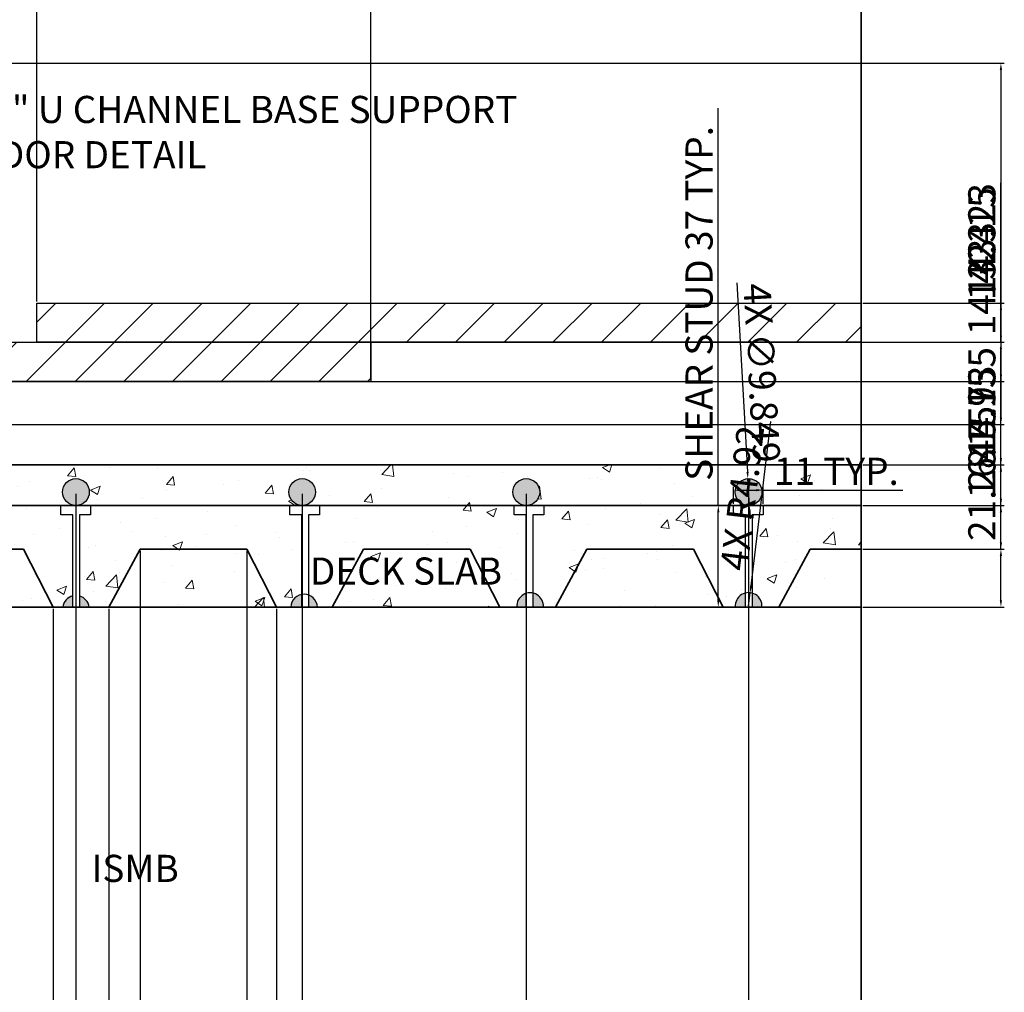
# Model space of a CAD drawing. Units: millimetres. Extents: x 1791 to 2420, y 1225 to 2361.
# Tile 3 of 4: x 2057 to 2420, y 1583 to 1941. Entities that reach past the tile are written whole.
import ezdxf
from ezdxf import colors
from ezdxf.entities.mleader import LeaderData, LeaderLine
from ezdxf.math import Vec2, Vec3

# ---------------------------------------------------------------- set-up
doc = ezdxf.new("R2010")
doc.units = ezdxf.units.MM
for name, color, linetype, lineweight in [('A-ANNO-DIMS', 2, 'Continuous', 18), ('A-ANNO-TEXT', 7, 'Continuous', 18), ('A-ANNO-TTLB', 7, 'Continuous', 35), ('A-DETL-PATT', 8, 'Continuous', 13), ('A-FLOR', 30, 'Continuous', 25), ('S-CONN', 6, 'Continuous', 25), ('S-DECK', 3, 'Continuous', 35)]:
    doc.layers.add(name, color=color, linetype=linetype, lineweight=lineweight)
doc.styles.get("Standard").update_dxf_attribs({"font": 'arial.ttf'})
doc.dimstyles.new('ISO-25', dxfattribs={"dimtxt": 10, "dimasz": 2.5, "dimexe": 1.25, "dimexo": 0.625, "dimtad": 1, "dimdec": 1, "dimtxsty": 'Standard', "dimcen": 2.5, "dimadec": 0, "dimazin": 0, "dimtfac": 1, "dimtdec": 1, "dimtmove": 0, "dimatfit": 3, "dimfxl": 1, "dimarcsym": 0})

# ---------------------------------------------------------------- blocks, each defined once
blk = doc.blocks.new('SHEAR-STUD')
for points in [[(4.38, 33.99), (0, 33.99), (0, 37.44), (10.9, 37.44), (10.9, 33.91), (6.86, 33.91)], [(6.86, 33.91), (6.86, 0), (4.38, 0), (4.38, 33.99)]]:
    blk.add_lwpolyline(points)
blk = doc.blocks.new('*D8')
at = {"layer": 'A-ANNO-DIMS', "color": 0, "lineweight": -2, "transparency": 16777216}
for p, q in [((2314.58, 1762.49), (2314.58, 1908.79)), ((2319.57, 1762.49), (2313.33, 1762.49)), ((2314.58, 1727.56), (2314.58, 1759.99)), ((2319.57, 1725.06), (2313.33, 1725.06))]:
    blk.add_line(p, q, dxfattribs=at)
at = {"layer": 'A-ANNO-DIMS', "color": 0, "transparency": 16777216}
for points in [[(2314.17, 1759.99), (2315, 1759.99), (2314.58, 1762.49)], [(2314.17, 1727.56), (2315, 1727.56), (2314.58, 1725.06)]]:
    blk.add_solid(points, dxfattribs=at)
at = {"layer": 'Defpoints', "color": 0, "transparency": 16777216}
for p in [(2314.58, 1762.49), (2320.2, 1762.49), (2320.2, 1725.06)]:
    blk.add_point(p, dxfattribs=at)
at = {"layer": 'A-ANNO-DIMS', "color": 0, "transparency": 16777216, "insert": (2308.78, 1836.89), "char_height": 10, "attachment_point": 5, "rotation": 90}
blk.add_mtext('SHEAR STUD 37 TYP.', dxfattribs=at)
blk = doc.blocks.new('*D9')
at = {"layer": 'A-ANNO-DIMS', "color": 0, "lineweight": -2, "transparency": 16777216}
for p, q in [((2320.2, 1763.12), (2320.2, 1769.36)), ((2322.7, 1768.11), (2328.6, 1768.11)), ((2331.1, 1763.12), (2331.1, 1769.36)), ((2331.1, 1768.11), (2382.58, 1768.11))]:
    blk.add_line(p, q, dxfattribs=at)
at = {"layer": 'A-ANNO-DIMS', "color": 0, "transparency": 16777216}
for points in [[(2322.7, 1768.52), (2322.7, 1767.69), (2320.2, 1768.11)], [(2328.6, 1768.52), (2328.6, 1767.69), (2331.1, 1768.11)]]:
    blk.add_solid(points, dxfattribs=at)
at = {"layer": 'Defpoints', "color": 0, "transparency": 16777216}
for p in [(2331.1, 1768.11), (2320.2, 1762.49), (2331.1, 1762.49)]:
    blk.add_point(p, dxfattribs=at)
at = {"layer": 'A-ANNO-DIMS', "color": 0, "transparency": 16777216, "insert": (2358.09, 1773.76), "char_height": 10, "attachment_point": 5}
blk.add_mtext('11 TYP.', dxfattribs=at)
blk = doc.blocks.new('*D18')
at = {"layer": 'A-ANNO-DIMS', "color": 0, "lineweight": -2, "transparency": 16777216}
for p, q in [((1926.15, 1925.42), (2419.97, 1925.42)), ((2418.72, 1922.92), (2418.72, 1794.77)), ((1926.15, 1792.27), (2419.97, 1792.27))]:
    blk.add_line(p, q, dxfattribs=at)
at = {"layer": 'A-ANNO-DIMS', "color": 0, "transparency": 16777216}
for points in [[(2418.3, 1922.92), (2419.13, 1922.92), (2418.72, 1925.42)], [(2418.3, 1794.77), (2419.13, 1794.77), (2418.72, 1792.27)]]:
    blk.add_solid(points, dxfattribs=at)
at = {"layer": 'Defpoints', "color": 0, "transparency": 16777216}
for p in [(1925.53, 1925.42), (1925.53, 1792.27), (2418.72, 1792.27)]:
    blk.add_point(p, dxfattribs=at)
at = {"layer": 'A-ANNO-DIMS', "color": 0, "transparency": 16777216, "insert": (2412.98, 1858.85), "char_height": 10, "attachment_point": 5, "rotation": 90}
blk.add_mtext('133.15', dxfattribs=at)
blk = doc.blocks.new('*D19')
at = {"layer": 'A-ANNO-DIMS', "color": 0, "lineweight": -2, "transparency": 16777216}
for p, q in [((2418.72, 1822.58), (2418.72, 1866.9)), ((1941, 1822.58), (2419.97, 1822.58)), ((2418.72, 1810.65), (2418.72, 1820.08)), ((1941, 1808.15), (2419.97, 1808.15))]:
    blk.add_line(p, q, dxfattribs=at)
at = {"layer": 'A-ANNO-DIMS', "color": 0, "transparency": 16777216}
for points in [[(2418.3, 1820.08), (2419.13, 1820.08), (2418.72, 1822.58)], [(2418.3, 1810.65), (2419.13, 1810.65), (2418.72, 1808.15)]]:
    blk.add_solid(points, dxfattribs=at)
at = {"layer": 'Defpoints', "color": 0, "transparency": 16777216}
for p in [(1940.38, 1822.58), (2418.72, 1822.58), (1940.38, 1808.15)]:
    blk.add_point(p, dxfattribs=at)
at = {"layer": 'A-ANNO-DIMS', "color": 0, "transparency": 16777216, "insert": (2412.98, 1845.99), "char_height": 10, "attachment_point": 5, "rotation": 90}
blk.add_mtext('14.423', dxfattribs=at)
blk = doc.blocks.new('*D22')
at = {"layer": 'A-ANNO-DIMS', "color": 0, "lineweight": -2, "transparency": 16777216}
for p, q in [((2418.72, 1746.33), (2418.72, 1784.02)), ((2367.84, 1746.33), (2419.97, 1746.33)), ((2418.72, 1727.56), (2418.72, 1743.83)), ((2367.84, 1725.06), (2419.97, 1725.06))]:
    blk.add_line(p, q, dxfattribs=at)
at = {"layer": 'A-ANNO-DIMS', "color": 0, "transparency": 16777216}
for points in [[(2418.3, 1743.83), (2419.13, 1743.83), (2418.72, 1746.33)], [(2418.3, 1727.56), (2419.13, 1727.56), (2418.72, 1725.06)]]:
    blk.add_solid(points, dxfattribs=at)
at = {"layer": 'Defpoints', "color": 0, "transparency": 16777216}
for p in [(2367.22, 1746.33), (2418.72, 1746.33), (2367.22, 1725.06)]:
    blk.add_point(p, dxfattribs=at)
at = {"layer": 'A-ANNO-DIMS', "color": 0, "transparency": 16777216, "insert": (2412.99, 1766.43), "char_height": 10, "attachment_point": 5, "rotation": 90}
blk.add_mtext('21.28', dxfattribs=at)
blk = doc.blocks.new('*D23')
at = {"layer": 'A-ANNO-DIMS', "color": 0, "lineweight": -2, "transparency": 16777216}
for p, q in [((2418.72, 1762.49), (2418.72, 1806.81)), ((2367.84, 1762.49), (2419.97, 1762.49)), ((2418.72, 1748.83), (2418.72, 1759.99)), ((2367.84, 1746.33), (2419.97, 1746.33))]:
    blk.add_line(p, q, dxfattribs=at)
at = {"layer": 'A-ANNO-DIMS', "color": 0, "transparency": 16777216}
for points in [[(2418.3, 1759.99), (2419.13, 1759.99), (2418.72, 1762.49)], [(2418.3, 1748.83), (2419.13, 1748.83), (2418.72, 1746.33)]]:
    blk.add_solid(points, dxfattribs=at)
at = {"layer": 'Defpoints', "color": 0, "transparency": 16777216}
for p in [(2367.22, 1762.49), (2418.72, 1762.49), (2367.22, 1746.33)]:
    blk.add_point(p, dxfattribs=at)
at = {"layer": 'A-ANNO-DIMS', "color": 0, "transparency": 16777216, "insert": (2412.99, 1785.9), "char_height": 10, "attachment_point": 5, "rotation": 90}
blk.add_mtext('16.157', dxfattribs=at)
blk = doc.blocks.new('*D24')
at = {"layer": 'A-ANNO-DIMS', "color": 0, "lineweight": -2, "transparency": 16777216}
for p, q in [((2418.72, 1777.42), (2418.72, 1813.97)), ((2367.84, 1777.42), (2419.97, 1777.42)), ((2418.72, 1764.99), (2418.72, 1774.92)), ((2367.84, 1762.49), (2419.97, 1762.49))]:
    blk.add_line(p, q, dxfattribs=at)
at = {"layer": 'A-ANNO-DIMS', "color": 0, "transparency": 16777216}
for points in [[(2418.3, 1774.92), (2419.13, 1774.92), (2418.72, 1777.42)], [(2418.3, 1764.99), (2419.13, 1764.99), (2418.72, 1762.49)]]:
    blk.add_solid(points, dxfattribs=at)
at = {"layer": 'Defpoints', "color": 0, "transparency": 16777216}
for p in [(2367.22, 1777.42), (2418.72, 1777.42), (2367.22, 1762.49)]:
    blk.add_point(p, dxfattribs=at)
at = {"layer": 'A-ANNO-DIMS', "color": 0, "transparency": 16777216, "insert": (2412.98, 1796.95), "char_height": 10, "attachment_point": 5, "rotation": 90}
blk.add_mtext('14.93', dxfattribs=at)
blk = doc.blocks.new('*D25')
at = {"layer": 'A-ANNO-DIMS', "color": 0, "lineweight": -2, "transparency": 16777216}
for p, q in [((2367.84, 1822.58), (2419.97, 1822.58)), ((2418.72, 1779.92), (2418.72, 1820.08)), ((2367.84, 1777.42), (2419.97, 1777.42))]:
    blk.add_line(p, q, dxfattribs=at)
at = {"layer": 'A-ANNO-DIMS', "color": 0, "transparency": 16777216}
for points in [[(2418.3, 1820.08), (2419.13, 1820.08), (2418.72, 1822.58)], [(2418.3, 1779.92), (2419.13, 1779.92), (2418.72, 1777.42)]]:
    blk.add_solid(points, dxfattribs=at)
at = {"layer": 'Defpoints', "color": 0, "transparency": 16777216}
for p in [(2367.22, 1822.58), (2418.72, 1822.58), (2367.22, 1777.42)]:
    blk.add_point(p, dxfattribs=at)
at = {"layer": 'A-ANNO-DIMS', "color": 0, "transparency": 16777216, "insert": (2412.99, 1800), "char_height": 10, "attachment_point": 5, "rotation": 90}
blk.add_mtext('45.155', dxfattribs=at)
blk = doc.blocks.new('*D26')
at = {"layer": 'A-ANNO-DIMS', "color": 0, "lineweight": -2, "transparency": 16777216}
for p, q in [((2418.72, 1837), (2418.72, 1881.32)), ((2367.84, 1837), (2419.97, 1837)), ((2418.72, 1825.08), (2418.72, 1834.5)), ((2367.84, 1822.58), (2419.97, 1822.58))]:
    blk.add_line(p, q, dxfattribs=at)
at = {"layer": 'A-ANNO-DIMS', "color": 0, "transparency": 16777216}
for points in [[(2418.3, 1834.5), (2419.13, 1834.5), (2418.72, 1837)], [(2418.3, 1825.08), (2419.13, 1825.08), (2418.72, 1822.58)]]:
    blk.add_solid(points, dxfattribs=at)
at = {"layer": 'Defpoints', "color": 0, "transparency": 16777216}
for p in [(2367.22, 1837), (2418.72, 1837), (2367.22, 1822.58)]:
    blk.add_point(p, dxfattribs=at)
at = {"layer": 'A-ANNO-DIMS', "color": 0, "transparency": 16777216, "insert": (2412.98, 1860.41), "char_height": 10, "attachment_point": 5, "rotation": 90}
blk.add_mtext('14.423', dxfattribs=at)
blk = doc.blocks.new('*D27')
at = {"layer": 'A-ANNO-DIMS', "color": 0, "lineweight": -2, "transparency": 16777216}
for p, q in [((1940.38, 1808.78), (1940.38, 2350.12)), ((1942.88, 2348.87), (2184.03, 2348.87)), ((2186.53, 1808.78), (2186.53, 2350.12))]:
    blk.add_line(p, q, dxfattribs=at)
at = {"layer": 'A-ANNO-DIMS', "color": 0, "transparency": 16777216}
for points in [[(1942.88, 2349.29), (1942.88, 2348.45), (1940.38, 2348.87)], [(2184.03, 2349.29), (2184.03, 2348.45), (2186.53, 2348.87)]]:
    blk.add_solid(points, dxfattribs=at)
at = {"layer": 'Defpoints', "color": 0, "transparency": 16777216}
for p in [(2186.53, 2348.87), (1940.38, 1808.15), (2186.53, 1808.15)]:
    blk.add_point(p, dxfattribs=at)
at = {"layer": 'A-ANNO-DIMS', "color": 0, "transparency": 16777216, "insert": (2063.45, 2354.6), "char_height": 10, "attachment_point": 5}
blk.add_mtext('246.15', dxfattribs=at)
blk = doc.blocks.new('*D28')
at = {"layer": 'A-ANNO-DIMS', "color": 0, "lineweight": -2, "transparency": 16777216}
for p, q in [((2063.45, 1837.62), (2063.45, 2350.12)), ((2065.95, 2348.87), (2364.72, 2348.87)), ((2367.22, 1837.62), (2367.22, 2350.12))]:
    blk.add_line(p, q, dxfattribs=at)
at = {"layer": 'A-ANNO-DIMS', "color": 0, "transparency": 16777216}
for points in [[(2065.95, 2349.29), (2065.95, 2348.45), (2063.45, 2348.87)], [(2364.72, 2349.29), (2364.72, 2348.45), (2367.22, 2348.87)]]:
    blk.add_solid(points, dxfattribs=at)
at = {"layer": 'Defpoints', "color": 0, "transparency": 16777216}
for p in [(2367.22, 2348.87), (2063.45, 1837), (2367.22, 1837)]:
    blk.add_point(p, dxfattribs=at)
at = {"layer": 'A-ANNO-DIMS', "color": 0, "transparency": 16777216, "insert": (2215.34, 2354.6), "char_height": 10, "attachment_point": 5}
blk.add_mtext('303.76', dxfattribs=at)
blk = doc.blocks.new('*D29')
at = {"layer": 'A-ANNO-DIMS', "color": 0, "lineweight": -2, "transparency": 16777216}
for p, q in [((2069.49, 1724.43), (2069.49, 1262.67)), ((2089.99, 1724.43), (2089.99, 1262.67)), ((2071.99, 1263.92), (2087.49, 1263.92)), ((2089.99, 1263.92), (2135.5, 1263.92))]:
    blk.add_line(p, q, dxfattribs=at)
at = {"layer": 'A-ANNO-DIMS', "color": 0, "transparency": 16777216}
for points in [[(2071.99, 1264.34), (2071.99, 1263.5), (2069.49, 1263.92)], [(2087.49, 1264.34), (2087.49, 1263.5), (2089.99, 1263.92)]]:
    blk.add_solid(points, dxfattribs=at)
at = {"layer": 'Defpoints', "color": 0, "transparency": 16777216}
for p in [(2069.49, 1725.06), (2089.99, 1725.06), (2089.99, 1263.92)]:
    blk.add_point(p, dxfattribs=at)
at = {"layer": 'A-ANNO-DIMS', "color": 0, "transparency": 16777216, "insert": (2113.99, 1269.65), "char_height": 10, "attachment_point": 5}
blk.add_mtext('20.495', dxfattribs=at)
blk = doc.blocks.new('*D30')
at = {"layer": 'A-ANNO-DIMS', "color": 0, "lineweight": -2, "transparency": 16777216}
for p, q in [((2069.49, 1724.43), (2069.49, 1262.67)), ((2151.78, 1724.43), (2151.78, 1262.67)), ((2071.99, 1263.92), (2149.28, 1263.92))]:
    blk.add_line(p, q, dxfattribs=at)
at = {"layer": 'A-ANNO-DIMS', "color": 0, "transparency": 16777216}
for points in [[(2071.99, 1264.34), (2071.99, 1263.5), (2069.49, 1263.92)], [(2149.28, 1264.34), (2149.28, 1263.5), (2151.78, 1263.92)]]:
    blk.add_solid(points, dxfattribs=at)
at = {"layer": 'Defpoints', "color": 0, "transparency": 16777216}
for p in [(2069.49, 1725.06), (2151.78, 1725.06), (2151.78, 1263.92)]:
    blk.add_point(p, dxfattribs=at)
at = {"layer": 'A-ANNO-DIMS', "color": 0, "transparency": 16777216, "insert": (2110.64, 1269.65), "char_height": 10, "attachment_point": 5}
blk.add_mtext('82.3', dxfattribs=at)
blk = doc.blocks.new('*D31')
at = {"layer": 'A-ANNO-DIMS', "color": 0, "lineweight": -2, "transparency": 16777216}
for p, q in [((2101.6, 1745.71), (2101.6, 1262.67)), ((2140.84, 1745.71), (2140.84, 1262.67)), ((2104.1, 1263.92), (2138.34, 1263.92))]:
    blk.add_line(p, q, dxfattribs=at)
at = {"layer": 'A-ANNO-DIMS', "color": 0, "transparency": 16777216}
for points in [[(2104.1, 1264.34), (2104.1, 1263.5), (2101.6, 1263.92)], [(2138.34, 1264.34), (2138.34, 1263.5), (2140.84, 1263.92)]]:
    blk.add_solid(points, dxfattribs=at)
at = {"layer": 'Defpoints', "color": 0, "transparency": 16777216}
for p in [(2101.6, 1746.33), (2140.84, 1746.33), (2140.84, 1263.92)]:
    blk.add_point(p, dxfattribs=at)
at = {"layer": 'A-ANNO-DIMS', "color": 0, "transparency": 16777216, "insert": (2121.22, 1269.65), "char_height": 10, "attachment_point": 5}
blk.add_mtext('39.24', dxfattribs=at)
blk = doc.blocks.new('*D32')
at = {"layer": 'A-ANNO-DIMS', "color": 0, "lineweight": -2, "transparency": 16777216}
for p, q in [((2077.9, 1766.79), (2077.9, 1262.67)), ((1953.66, 1761.87), (1953.66, 1262.67)), ((1956.16, 1263.92), (2075.4, 1263.92))]:
    blk.add_line(p, q, dxfattribs=at)
at = {"layer": 'A-ANNO-DIMS', "color": 0, "transparency": 16777216}
for points in [[(1956.16, 1264.34), (1956.16, 1263.5), (1953.66, 1263.92)], [(2075.4, 1264.34), (2075.4, 1263.5), (2077.9, 1263.92)]]:
    blk.add_solid(points, dxfattribs=at)
at = {"layer": 'Defpoints', "color": 0, "transparency": 16777216}
for p in [(2077.9, 1767.42), (1953.66, 1762.49), (2077.9, 1263.92)]:
    blk.add_point(p, dxfattribs=at)
at = {"layer": 'A-ANNO-DIMS', "color": 0, "transparency": 16777216, "insert": (2015.78, 1269.57), "char_height": 10, "attachment_point": 5}
blk.add_mtext('124.24', dxfattribs=at)
blk = doc.blocks.new('*D33')
at = {"layer": 'A-ANNO-DIMS', "color": 0, "lineweight": -2, "transparency": 16777216}
for p, q in [((2077.9, 1766.79), (2077.9, 1262.67)), ((2161.26, 1766.79), (2161.26, 1262.67)), ((2080.4, 1263.92), (2158.76, 1263.92))]:
    blk.add_line(p, q, dxfattribs=at)
at = {"layer": 'A-ANNO-DIMS', "color": 0, "transparency": 16777216}
for points in [[(2080.4, 1264.34), (2080.4, 1263.5), (2077.9, 1263.92)], [(2158.76, 1264.34), (2158.76, 1263.5), (2161.26, 1263.92)]]:
    blk.add_solid(points, dxfattribs=at)
at = {"layer": 'Defpoints', "color": 0, "transparency": 16777216}
for p in [(2077.9, 1767.42), (2161.26, 1767.42), (2161.26, 1263.92)]:
    blk.add_point(p, dxfattribs=at)
at = {"layer": 'A-ANNO-DIMS', "color": 0, "transparency": 16777216, "insert": (2119.58, 1269.65), "char_height": 10, "attachment_point": 5}
blk.add_mtext('83.36', dxfattribs=at)
blk = doc.blocks.new('*D34')
at = {"layer": 'A-ANNO-DIMS', "color": 0, "lineweight": -2, "transparency": 16777216}
for p, q in [((2161.26, 1766.79), (2161.26, 1262.67)), ((2243.84, 1766.79), (2243.84, 1262.67)), ((2163.76, 1263.92), (2241.34, 1263.92))]:
    blk.add_line(p, q, dxfattribs=at)
at = {"layer": 'A-ANNO-DIMS', "color": 0, "transparency": 16777216}
for points in [[(2163.76, 1264.34), (2163.76, 1263.5), (2161.26, 1263.92)], [(2241.34, 1264.34), (2241.34, 1263.5), (2243.84, 1263.92)]]:
    blk.add_solid(points, dxfattribs=at)
at = {"layer": 'Defpoints', "color": 0, "transparency": 16777216}
for p in [(2161.26, 1767.42), (2243.84, 1767.42), (2243.84, 1263.92)]:
    blk.add_point(p, dxfattribs=at)
at = {"layer": 'A-ANNO-DIMS', "color": 0, "transparency": 16777216, "insert": (2202.55, 1269.65), "char_height": 10, "attachment_point": 5}
blk.add_mtext('82.58', dxfattribs=at)
blk = doc.blocks.new('*D35')
at = {"layer": 'A-ANNO-DIMS', "color": 0, "lineweight": -2, "transparency": 16777216}
for p, q in [((2243.84, 1766.79), (2243.84, 1262.67)), ((2325.75, 1766.79), (2325.75, 1262.67)), ((2246.34, 1263.92), (2323.25, 1263.92))]:
    blk.add_line(p, q, dxfattribs=at)
at = {"layer": 'A-ANNO-DIMS', "color": 0, "transparency": 16777216}
for points in [[(2246.34, 1264.34), (2246.34, 1263.5), (2243.84, 1263.92)], [(2323.25, 1264.34), (2323.25, 1263.5), (2325.75, 1263.92)]]:
    blk.add_solid(points, dxfattribs=at)
at = {"layer": 'Defpoints', "color": 0, "transparency": 16777216}
for p in [(2243.84, 1767.42), (2325.75, 1767.42), (2325.75, 1263.92)]:
    blk.add_point(p, dxfattribs=at)
at = {"layer": 'A-ANNO-DIMS', "color": 0, "transparency": 16777216, "insert": (2284.8, 1269.65), "char_height": 10, "attachment_point": 5}
blk.add_mtext('81.92', dxfattribs=at)
blk = doc.blocks.new('*D42')
at = {"layer": 'A-ANNO-DIMS', "color": 0, "lineweight": -2, "transparency": 16777216}
for p, q in [((2321.47, 1844.47), (2325.34, 1774.83)), ((2326.03, 1762.5), (2325.48, 1772.33)), ((2326.17, 1760), (2326.31, 1757.51))]:
    blk.add_line(p, q, dxfattribs=at)
at = {"layer": 'A-ANNO-DIMS', "color": 0, "transparency": 16777216}
for points in [[(2325.76, 1774.85), (2324.93, 1774.81), (2325.48, 1772.33)], [(2326.58, 1760.03), (2325.75, 1759.98), (2326.03, 1762.5)]]:
    blk.add_solid(points, dxfattribs=at)
at = {"layer": 'Defpoints', "color": 0, "transparency": 16777216}
for p in [(2325.48, 1772.33), (2326.03, 1762.5)]:
    blk.add_point(p, dxfattribs=at)
at = {"layer": 'A-ANNO-DIMS', "color": 0, "transparency": 16777216, "insert": (2329.34, 1811.23), "char_height": 10, "attachment_point": 5, "rotation": 273.1821}
blk.add_mtext('4X ∅9.849', dxfattribs=at)
blk = doc.blocks.new('*D43')
at = {"layer": 'A-ANNO-DIMS', "color": 0, "lineweight": -2, "transparency": 16777216}
for p, q in [((2333.86, 1793.46), (2326.63, 1732.81)), ((2325.76, 1725.44), (2326.34, 1730.33))]:
    blk.add_line(p, q, dxfattribs=at)
at = {"layer": 'A-ANNO-DIMS', "color": 0, "transparency": 16777216}
blk.add_solid([(2326.22, 1732.86), (2327.05, 1732.76), (2326.34, 1730.33)], dxfattribs=at)
at = {"layer": 'Defpoints', "color": 0, "transparency": 16777216}
for p in [(2326.34, 1730.33), (2325.76, 1725.44)]:
    blk.add_point(p, dxfattribs=at)
at = {"layer": 'A-ANNO-DIMS', "color": 0, "transparency": 16777216, "insert": (2324.7, 1765.06), "char_height": 10, "attachment_point": 5, "rotation": 83.2097}
blk.add_mtext('4X R4.92', dxfattribs=at)

msp = doc.modelspace()

# ---------------------------------------------------------------- hatches: boundary and pattern name
at = {"layer": 'A-DETL-PATT'}
h = msp.add_hatch(dxfattribs=at)
h.set_pattern_fill('ANSI31', color=256, scale=4)
h.paths.add_polyline_path([(2186.5283, 1822.576), (2063.4532, 1822.576), (1940.378, 1822.576), (1940.378, 1808.1531), (2186.5283, 1808.1531)])
h.paths.add_polyline_path([(2367.2176, 1836.999), (2063.4532, 1836.999), (2063.4532, 1822.576), (2367.2176, 1822.576)])
h = msp.add_hatch(dxfattribs=at)
h.set_pattern_fill('AR-CONC', color=256, scale=0.2)
h.paths.add_polyline_path([(2058.5452, 1746.3347), (2035.8237, 1746.3347), (2030.2178, 1746.3347), (2016.5047, 1746.3347), (2004.8892, 1725.0563), (2069.4909, 1725.0563)], flags=17)
h.paths.add_polyline_path([(2166.1796, 1767.4162, -0.41421356), (2161.2551, 1762.4917), (2167.6174, 1762.4917), (2243.8358, 1762.4917, -0.41421356), (2238.9113, 1767.4162, -1), (2248.7603, 1767.4162, -0.41421356), (2243.8358, 1762.4917), (2250.3259, 1762.4917), (2325.7548, 1762.4917, -0.41421356), (2320.8303, 1767.4162, -1), (2330.6793, 1767.4162, -0.41421356), (2325.7548, 1762.4917), (2331.0978, 1762.4917), (2367.2176, 1762.4917), (2367.2176, 1777.4206), (2034.727, 1777.4206), (2034.727, 1770.4206, -0.41421356), (2029.727, 1765.4206), (1960.727, 1765.4206, 0.19891237), (1953.6559, 1762.4917), (2077.8995, 1762.4917, -0.41421356), (2072.975, 1767.4162, -1), (2082.824, 1767.4162, -0.41421356), (2077.8995, 1762.4917), (2083.2584, 1762.4917), (2161.2551, 1762.4917, -0.41421356), (2156.3306, 1767.4162, -1)])
h.paths.add_polyline_path([(2016.5047, 1746.3347), (2030.2178, 1746.3347), (2035.8237, 1746.3347), (2058.5452, 1746.3347), (2069.4909, 1725.0563), (2073.0274, 1725.0563, -0.30569965), (2076.7379, 1729.1256), (2076.7379, 1759.0444), (2072.3578, 1759.0444), (2072.3578, 1762.4917), (1953.6559, 1762.4917, 0.19891237), (1950.727, 1755.4206), (1950.727, 1746.3347), (1973.4485, 1746.3347), (1984.3943, 1725.0563), (2004.8892, 1725.0563)])
h.paths.add_polyline_path([(1973.4485, 1746.3347), (1950.727, 1746.3347), (1950.727, 1725.0563), (1984.3943, 1725.0563)], flags=17)
h.paths.add_polyline_path([(2140.839, 1746.3347), (2118.1174, 1746.3347), (2115.3145, 1746.3347), (2101.6014, 1746.3347), (2089.9858, 1725.0563), (2151.7847, 1725.0563)], flags=17)
h.paths.add_polyline_path([(2161.0969, 1759.0444), (2156.7168, 1759.0444), (2156.7168, 1762.4917), (2083.2584, 1762.4917), (2083.2584, 1758.968), (2079.2222, 1758.968), (2079.2222, 1729.0836, -0.29648266), (2082.7716, 1725.0563), (2089.9858, 1725.0563), (2101.6014, 1746.3347), (2115.3145, 1746.3347), (2120.9204, 1746.3347), (2140.839, 1746.3347), (2151.7847, 1725.0563), (2157.0332, 1725.0563, -0.35098402), (2161.0969, 1729.6797)])
h.paths.add_polyline_path([(2243.8053, 1759.0444), (2239.4253, 1759.0444), (2239.4253, 1762.4917), (2167.6174, 1762.4917), (2167.6174, 1758.968), (2163.5811, 1758.968), (2163.5811, 1729.4775, -0.30598924), (2166.8718, 1725.0563), (2172.2796, 1725.0563), (2183.8952, 1746.3347), (2197.6083, 1746.3347), (2203.2141, 1746.3347), (2223.1327, 1746.3347), (2234.0785, 1725.0563), (2240.3204, 1725.0563, -0.34708966), (2243.8053, 1730.0651)])
h.paths.add_polyline_path([(2223.1327, 1746.3347), (2200.4112, 1746.3347), (2197.6083, 1746.3347), (2183.8952, 1746.3347), (2172.2796, 1725.0563), (2234.0785, 1725.0563)], flags=17)
h.paths.add_polyline_path([(2324.5773, 1759.0444), (2320.1972, 1759.0444), (2320.1972, 1762.4917), (2250.3259, 1762.4917), (2250.3259, 1758.968), (2246.2896, 1758.968), (2246.2896, 1730.1635, -0.36941305), (2250.1515, 1725.0563), (2254.5734, 1725.0563), (2266.1889, 1746.3347), (2279.902, 1746.3347), (2285.5079, 1746.3347), (2305.4265, 1746.3347), (2316.3722, 1725.0563), (2320.8471, 1725.0563, -0.36687812), (2324.5773, 1730.2193)])
h.paths.add_polyline_path([(2305.4265, 1746.3347), (2282.705, 1746.3347), (2279.902, 1746.3347), (2266.1889, 1746.3347), (2254.5734, 1725.0563), (2316.3722, 1725.0563)], flags=17)
h.paths.add_polyline_path([(2367.2176, 1762.4917), (2331.0978, 1762.4917), (2331.0978, 1758.968), (2327.0615, 1758.968), (2327.0615, 1730.1866, -0.3594453), (2330.6665, 1725.0563), (2336.8671, 1725.0563), (2348.4827, 1746.3347), (2362.1958, 1746.3347), (2367.2176, 1746.3347)])
h.paths.add_polyline_path([(2367.2176, 1746.3347), (2362.1958, 1746.3347), (2348.4827, 1746.3347), (2336.8671, 1725.0563), (2367.2176, 1725.0563)], flags=17)
h = msp.add_hatch(color=256, dxfattribs=at)
h.dxf.hatch_style = 1
h.paths.add_polyline_path([(2082.824, 1767.4162, 1), (2072.975, 1767.4162, 1)])
h.paths.add_polyline_path([(2156.3306, 1767.4162, 1), (2166.1796, 1767.4162, 1)])
h.paths.add_polyline_path([(2248.7603, 1767.4162, 1), (2238.9113, 1767.4162, 1)])
h.paths.add_polyline_path([(2330.6793, 1767.4162, 1), (2320.8303, 1767.4162, 1)])
h.paths.add_polyline_path([(2324.5773, 1730.2193, 0.36687812), (2320.8471, 1725.0563), (2324.5773, 1725.0563)])
h.paths.add_polyline_path([(2327.0615, 1730.1866), (2327.0615, 1725.0563), (2330.6665, 1725.0563, 0.3594453)])
h.paths.add_polyline_path([(2243.8053, 1730.0651, 0.34708966), (2240.3204, 1725.0563), (2243.8053, 1725.0563)])
h.paths.add_polyline_path([(2246.2896, 1730.1635), (2246.2896, 1725.0563), (2250.1515, 1725.0563, 0.36941305)])
h.paths.add_polyline_path([(2161.0969, 1729.6797, 0.35098402), (2157.0332, 1725.0563), (2161.0969, 1725.0563)])
h.paths.add_polyline_path([(2163.5811, 1729.4775), (2163.5811, 1725.0563), (2166.8718, 1725.0563, 0.30598924)])
h.paths.add_polyline_path([(2076.7379, 1729.1256, 0.30569965), (2073.0274, 1725.0563), (2076.7379, 1725.0563)])
h.paths.add_polyline_path([(2079.2222, 1729.0836), (2079.2222, 1725.0563), (2082.7716, 1725.0563, 0.29648266)])

# ---------------------------------------------------------------- linework, layer by layer
at = {"layer": 'A-ANNO-TTLB'}
msp.add_line((2367.2176, 2307.8191), (2367.2176, 1287.0028), dxfattribs=at)
at = {"layer": 'A-FLOR'}
for points in [[(2063.4532, 1836.999), (2367.2176, 1836.999), (2367.2176, 1822.576), (2063.4532, 1822.576)], [(1940.378, 1822.576), (2186.5283, 1822.576), (2186.5283, 1808.1531), (1940.378, 1808.1531)]]:
    msp.add_lwpolyline(points, close=True, dxfattribs=at)
at = {"layer": 'S-CONN'}
for centre in [(2077.8995, 1767.4162), (2161.2551, 1767.4162), (2243.8358, 1767.4162), (2325.7548, 1767.4162)]:
    msp.add_circle(centre, 4.9245, dxfattribs=at)
for centre, start, end in [((2077.8995, 1724.3401), 103.643637, 171.637133), ((2077.8995, 1724.3401), 8.362867, 74.419575), ((2161.9525, 1724.8301), 2.633093, 177.366907), ((2245.236, 1725.353), 356.545909, 183.454091), ((2325.7568, 1725.4381), 355.553377, 184.446623)]:
    msp.add_arc(centre, 4.9245, start, end, dxfattribs=at)
at = {"layer": 'S-DECK'}
for p, q in [((1854.727, 1777.4206), (2367.2176, 1777.4206)), ((1953.6559, 1762.4917), (2367.2176, 1762.4917)), ((1950.727, 1725.0563), (2367.2176, 1725.0563))]:
    msp.add_line(p, q, dxfattribs=at)
for points in [[(2035.8237, 1746.3347), (2058.5452, 1746.3347), (2069.4909, 1725.0563), (2089.9858, 1725.0563), (2101.6014, 1746.3347), (2115.3145, 1746.3347), (2120.9204, 1746.3347)], [(2118.1174, 1746.3347), (2140.839, 1746.3347), (2151.7847, 1725.0563), (2172.2796, 1725.0563), (2183.8952, 1746.3347), (2197.6083, 1746.3347), (2203.2141, 1746.3347)], [(2200.4112, 1746.3347), (2223.1327, 1746.3347), (2234.0785, 1725.0563), (2254.5734, 1725.0563), (2266.1889, 1746.3347), (2279.902, 1746.3347), (2285.5079, 1746.3347)], [(2282.705, 1746.3347), (2305.4265, 1746.3347), (2316.3722, 1725.0563), (2336.8671, 1725.0563), (2348.4827, 1746.3347), (2362.1958, 1746.3347), (2367.2176, 1746.3347)]]:
    msp.add_lwpolyline(points, dxfattribs=at)

# ---------------------------------------------------------------- block references
at = {"layer": 'S-CONN'}
for p in [(2072.358, 1725.056), (2156.7169, 1725.056), (2239.4254, 1725.056), (2320.1973, 1725.056)]:
    msp.add_blockref('SHEAR-STUD', p, dxfattribs=at)

# ---------------------------------------------------------------- texts
at = {"layer": 'A-ANNO-TEXT', "char_height": 10, "attachment_point": 1}
for s, width, insert in [('{\\fArial|b1|i0|c0|p34;DECK SLAB}', 84.955679, (2164.0983, 1743.2967)), ('ISMB', 111.201462, (2083.6179, 1633.7629))]:
    msp.add_mtext_dynamic_manual_height_columns(s, width=width, gutter_width=12.5, heights=[0], dxfattribs=dict(at, insert=insert))

# ---------------------------------------------------------------- dimensions: what is measured, and where the dimension line sits
at = {"layer": 'A-ANNO-DIMS'}
for base, p1, p2, override, picture, middle in [((2186.5283, 2348.8684), (1940.378, 1808.1531), (2186.5283, 1808.1531), {"dimdec": 2, "dimlfac": 1, "dimrnd": 0, "dimzin": 0, "dimdsep": 46, "dimlunit": 2}, '*D27', (2063.4532, 2354.5991)), ((2367.2176, 2348.8684), (2063.4532, 1836.999), (2367.2176, 1836.999), {"dimdec": 2, "dimlfac": 1, "dimrnd": 0, "dimzin": 0, "dimdsep": 46, "dimlunit": 2}, '*D28', (2215.3354, 2354.6025)), ((2077.8995, 1263.9206), (1953.6559, 1762.4917), (2077.8995, 1767.4162), {"dimdec": 2, "dimlfac": 1, "dimrnd": 0, "dimzin": 0, "dimdsep": 46, "dimlunit": 2}, '*D32', (2015.7777, 1269.566)), ((2161.2551, 1263.9206), (2077.8995, 1767.4162), (2161.2551, 1767.4162), {"dimdec": 2, "dimlfac": 1, "dimrnd": 0, "dimzin": 0, "dimdsep": 46, "dimlunit": 2}, '*D33', (2119.5773, 1269.6547)), ((2243.8358, 1263.9206), (2161.2551, 1767.4162), (2243.8358, 1767.4162), {"dimdec": 2, "dimlfac": 1, "dimrnd": 0, "dimzin": 0, "dimdsep": 46, "dimlunit": 2}, '*D34', (2202.5454, 1269.6513)), ((2325.7548, 1263.9206), (2243.8358, 1767.4162), (2325.7548, 1767.4162), {"dimdec": 2, "dimlfac": 1, "dimrnd": 0, "dimzin": 0, "dimdsep": 46, "dimlunit": 2}, '*D35', (2284.7953, 1269.6513)), ((2140.839, 1263.9206), (2101.6014, 1746.3347), (2140.839, 1746.3347), {"dimdec": 2, "dimlfac": 1, "dimrnd": 0, "dimzin": 0, "dimdsep": 46, "dimlunit": 2}, '*D31', (2121.2202, 1269.6547)), ((2089.9858, 1263.9206), (2069.4909, 1725.0563), (2089.9858, 1725.0563), {"dimdec": 3, "dimlfac": 1, "dimrnd": 0, "dimzin": 0, "dimdsep": 46, "dimlunit": 2}, '*D29', (2113.9908, 1269.6513)), ((2151.7847, 1263.9206), (2069.4909, 1725.0563), (2151.7847, 1725.0563), {"dimdec": 1, "dimlfac": 1, "dimrnd": 0, "dimzin": 0, "dimdsep": 46, "dimlunit": 2}, '*D30', (2110.6378, 1269.6547))]:
    dim = msp.add_linear_dim(base=base, p1=p1, p2=p2, dimstyle='ISO-25', override=override, dxfattribs=at)
    dim.commit()
    dim.dimension.update_dxf_attribs({"geometry": picture, "text_midpoint": middle})
for base, p1, p2, override, picture, middle in [((2418.7176, 1792.271), (1925.5277, 1925.4206), (1925.5277, 1792.271), {"dimdec": 2, "dimlfac": 1, "dimrnd": 0, "dimzin": 0, "dimdsep": 46, "dimlunit": 2}, '*D18', (2412.9835, 1858.8458)), ((2418.7176, 1836.999), (2367.2176, 1822.576), (2367.2176, 1836.999), {"dimdec": 3, "dimlfac": 1, "dimrnd": 0, "dimzin": 0, "dimdsep": 46, "dimlunit": 2}, '*D26', (2412.9835, 1860.4105)), ((2418.7176, 1822.576), (1940.378, 1808.1531), (1940.378, 1822.576), {"dimdec": 3, "dimlfac": 1, "dimrnd": 0, "dimzin": 0, "dimdsep": 46, "dimlunit": 2}, '*D19', (2412.9835, 1845.9875)), ((2418.7176, 1822.576), (2367.2176, 1777.4206), (2367.2176, 1822.576), {"dimdec": 3, "dimlfac": 1, "dimrnd": 0, "dimzin": 0, "dimdsep": 46, "dimlunit": 2}, '*D25', (2412.9869, 1799.9983)), ((2418.7176, 1777.4206), (2367.2176, 1762.4917), (2367.2176, 1777.4206), {"dimdec": 2, "dimlfac": 1, "dimrnd": 0, "dimzin": 0, "dimdsep": 46, "dimlunit": 2}, '*D24', (2412.9835, 1796.9474)), ((2418.7176, 1762.4917), (2367.2176, 1746.3347), (2367.2176, 1762.4917), {"dimdec": 3, "dimlfac": 1, "dimrnd": 0, "dimzin": 0, "dimdsep": 46, "dimlunit": 2}, '*D23', (2412.9869, 1785.9031)), ((2418.7176, 1746.3347), (2367.2176, 1725.0563), (2367.2176, 1746.3347), {"dimdec": 2, "dimlfac": 1, "dimrnd": 0, "dimzin": 0, "dimdsep": 46, "dimlunit": 2}, '*D22', (2412.9869, 1766.4277))]:
    dim = msp.add_linear_dim(base=base, p1=p1, p2=p2, angle=90, dimstyle='ISO-25', override=override, dxfattribs=at)
    dim.commit()
    dim.dimension.update_dxf_attribs({"geometry": picture, "text_midpoint": middle})
dim = msp.add_linear_dim(base=(2314.5819, 1762.4917), p1=(2320.1972, 1725.0563), p2=(2320.1972, 1762.4917), angle=90, text='SHEAR STUD <> TYP.', dimstyle='ISO-25', override={"dimdec": 0, "dimrnd": 0, "dimzin": 0, "dimlunit": 2}, dxfattribs=at)
dim.commit()
dim.dimension.update_dxf_attribs({"geometry": '*D8', "text_midpoint": (2308.7829, 1836.8922)})
dim = msp.add_diameter_dim_2p(p1=(2326.0282, 1762.4992), p2=(2325.4815, 1772.3331), text='4X <>', dimstyle='ISO-25', override={"dimdec": 3, "dimlfac": 1, "dimrnd": 0, "dimzin": 0, "dimdsep": 46, "dimlunit": 2}, dxfattribs=at)
dim.commit()
dim.dimension.update_dxf_attribs({"geometry": '*D42', "text_midpoint": (2323.3373, 1810.8999), "dimtype": 163})
dim = msp.add_radius_dim(center=(2325.7568, 1725.4381), mpoint=(2326.3391, 1730.3281), text='4X <>', dimstyle='ISO-25', override={"dimdec": 2, "dimlfac": 1, "dimrnd": 0, "dimzin": 0, "dimdsep": 46, "dimlunit": 2}, dxfattribs=at)
dim.commit()
dim.dimension.update_dxf_attribs({"geometry": '*D43', "text_midpoint": (2324.703, 1765.0566)})
dim = msp.add_linear_dim(base=(2331.0978, 1768.107), p1=(2320.1972, 1762.4917), p2=(2331.0978, 1762.4917), text='<> TYP.', dimstyle='ISO-25', override={"dimdec": 0, "dimrnd": 0, "dimzin": 0, "dimlunit": 2}, dxfattribs=at)
dim.commit()
dim.dimension.update_dxf_attribs({"geometry": '*D9', "text_midpoint": (2358.0905, 1773.7558)})

# ---------------------------------------------------------------- leaders
at = {"layer": 'A-ANNO-TEXT'}
ml = msp.add_multileader_mtext('Standard', dxfattribs=at)
ml.set_content('ALUMINIUM " U CHANNEL BASE SUPPORT\\PAS PER VENDOR DETAIL', color=256)
ml.set_leader_properties()
ml.build(insert=Vec2(0, 0))
ctx = ml.context
ctx.base_point, ctx.char_height, ctx.plane_origin = Vec3(1973.8617, 1908.272), 10, Vec3(1940.378, 1908.272)
notes = []
notes.append((ctx, [(0, (1, 1, 0), (1965.8617, 1908.272), (1, 0), 8, [(0, [(1940.378, 1908.272)], 0, [])])]))
ctx.mtext.insert, ctx.mtext.flow_direction = Vec3(1975.8617, 1913.3573), 5
for ctx, leaders in notes:
    for number, flags, end, landing, length, lines in leaders:
        leader = LeaderData()
        leader.index, (leader.has_last_leader_line, leader.has_dogleg_vector, leader.attachment_direction) = number, flags
        leader.last_leader_point, leader.dogleg_vector, leader.dogleg_length = Vec3(end), Vec3(landing), length
        for number, points, colour, breaks in lines:
            line = LeaderLine()
            line.index, line.vertices, line.color, line.breaks = number, Vec3.list(points), colors.encode_raw_color(colour), breaks
            leader.lines.append(line)
        ctx.leaders.append(leader)

doc.saveas('drawing.dxf')
